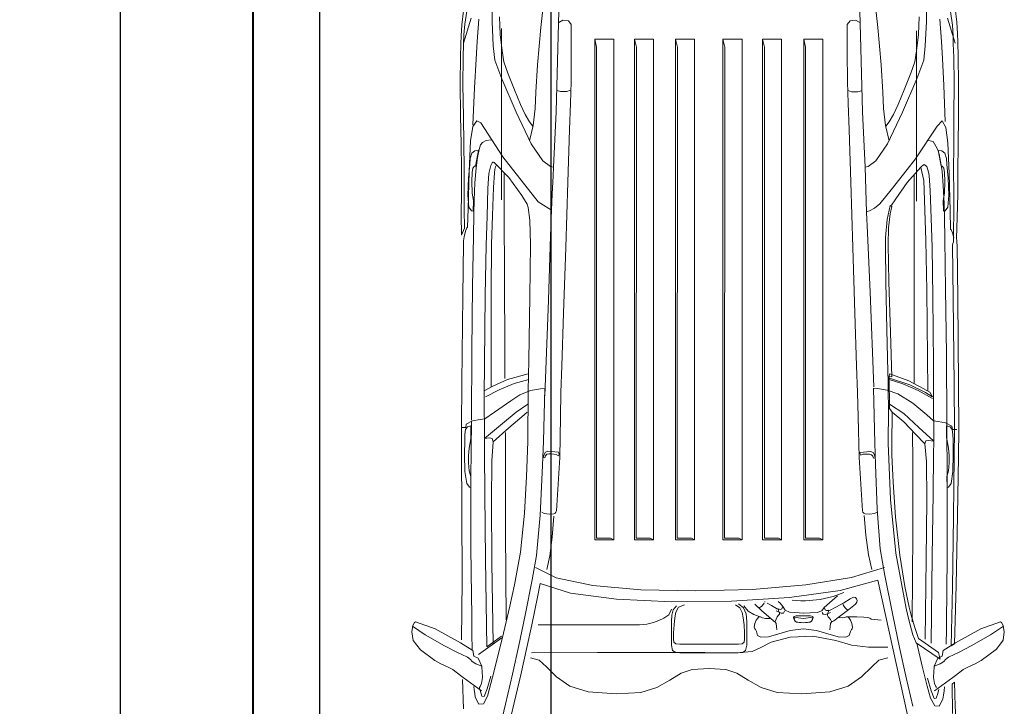
# Model space of a CAD drawing. Units: inches. Extents: x -19 to 419, y -828 to 43.
# Tile 2 of 9: x -9 to 124, y -720 to -627. Entities that reach past the tile are written whole.
import ezdxf

# ---------------------------------------------------------------- set-up
doc = ezdxf.new("R2010")
doc.units = ezdxf.units.IN
doc.header["$MEASUREMENT"] = 0
for name, color, linetype, lineweight in [('A-ANNO-DIMS', 2, 'Continuous', 18), ('A-EQPM-VEHI', 8, 'Continuous', 13), ('A-WALL', 7, 'Continuous', 40)]:
    doc.layers.add(name, color=color, linetype=linetype, lineweight=lineweight)
doc.styles.get("Standard").update_dxf_attribs({"font": 'arial.ttf'})
doc.dimstyles.get("Standard").update_dxf_attribs({"dimtxt": 0.18, "dimasz": 0.18, "dimexe": 0.18, "dimexo": 0.0625, "dimgap": 0.09, "dimtad": 0, "dimtih": 1, "dimtoh": 1, "dimdec": 0, "dimzin": 0, "dimdsep": 46, "dimlunit": 3, "dimtxsty": 'Standard', "dimcen": 0.09, "dimadec": 0, "dimazin": 0, "dimtfac": 1, "dimtdec": 0, "dimtofl": 0, "dimtmove": 0, "dimatfit": 3, "dimfxl": 1, "dimtolj": 1, "dimtzin": 0, "dimarcsym": 0})

# ---------------------------------------------------------------- blocks, each defined once
blk = doc.blocks.new('*D2')
at = {"layer": 'A-ANNO-DIMS', "color": 0, "lineweight": -2, "transparency": 16777216}
for p, q in [((22.68, 4.77), (4.74, 4.77)), ((4.92, 4.59), (4.92, -387.33)), ((4.92, -785.55), (4.92, -393.64)), ((22.68, -785.73), (4.74, -785.73))]:
    blk.add_line(p, q, dxfattribs=at)
at = {"layer": 'A-ANNO-DIMS', "color": 0, "transparency": 16777216}
for points in [[(4.89, 4.59), (4.95, 4.59), (4.92, 4.77)], [(4.89, -785.55), (4.95, -785.55), (4.92, -785.73)]]:
    blk.add_solid(points, dxfattribs=at)
at = {"layer": 'Defpoints', "color": 0, "transparency": 16777216}
for p in [(22.74, 4.77), (4.92, -785.73), (22.74, -785.73)]:
    blk.add_point(p, dxfattribs=at)
at = {"layer": 'A-ANNO-DIMS', "color": 0, "transparency": 16777216, "insert": (4.92, -390.48), "char_height": 6, "attachment_point": 5}
blk.add_mtext('\\A1;65\'-11"', dxfattribs=at)
blk = doc.blocks.new('*D49')
at = {"layer": 'A-ANNO-DIMS', "color": 0, "lineweight": -2, "transparency": 16777216}
for p, q in [((31.74, -574.3), (31.74, -827.51)), ((62.91, -574.3), (62.91, -827.51)), ((31.92, -827.33), (46.99, -827.33)), ((62.73, -827.33), (47.65, -827.33))]:
    blk.add_line(p, q, dxfattribs=at)
at = {"layer": 'A-ANNO-DIMS', "color": 0, "transparency": 16777216}
for points in [[(31.92, -827.3), (31.92, -827.36), (31.74, -827.33)], [(62.73, -827.3), (62.73, -827.36), (62.91, -827.33)]]:
    blk.add_solid(points, dxfattribs=at)
at = {"layer": 'Defpoints', "color": 0, "transparency": 16777216}
for p in [(31.74, -574.23), (62.91, -574.23), (62.91, -827.33)]:
    blk.add_point(p, dxfattribs=at)
at = {"layer": 'A-ANNO-DIMS', "color": 0, "transparency": 16777216, "insert": (47.32, -827.33), "char_height": 0.18, "attachment_point": 5}
blk.add_mtext('\\A1;2\'-7"', dxfattribs=at)

msp = doc.modelspace()

# ---------------------------------------------------------------- linework, layer by layer
at = {"layer": 'A-EQPM-VEHI'}
for p, q in [((55.01, -627.49), (55.03, -624.8)), ((113.5, -627.49), (113.48, -624.8)), ((50.91, -627.91), (51.15, -626.02)), ((51.59, -626.09), (51.31, -627.85)), ((61.53, -628.28), (61.9, -625.06)), ((63.86, -631.09), (63.96, -626.08)), ((104.65, -631.09), (104.55, -626.08)), ((106.97, -628.28), (106.61, -625.06)), ((117.01, -627.96), (116.77, -626.12)), ((117.37, -625.69), (117.61, -627.58)), ((51.11, -630.39), (52.17, -627.01)), ((52.97, -630.19), (53.18, -627.18)), ((55.15, -630.74), (55.01, -627.49)), ((56.07, -629.23), (55.99, -626.85)), ((63.96, -627.62), (64.51, -627.28)), ((64.51, -627.28), (65.27, -627.39)), ((65.27, -627.39), (65.65, -627.86)), ((103.22, -627.39), (102.84, -627.86)), ((103.97, -627.28), (103.22, -627.39)), ((104.52, -627.62), (103.97, -627.28)), ((112.44, -629.23), (112.51, -626.85)), ((113.35, -630.74), (113.5, -627.49)), ((115.53, -630.19), (115.32, -627.18)), ((117.4, -630.39), (116.34, -627.01)), ((50.81, -629.42), (50.91, -627.91)), ((51.31, -627.85), (51.19, -629.27)), ((56.23, -651.51), (56.23, -628.43)), ((61.11, -633.31), (61.53, -628.28)), ((65.65, -627.86), (65.65, -631.57)), ((102.84, -627.86), (102.84, -631.57)), ((107.4, -633.31), (106.97, -628.28)), ((112.17, -651.67), (112.17, -628.72)), ((117.1, -629.42), (117.01, -627.96)), ((117.61, -627.58), (117.71, -629.09)), ((50.78, -630.5), (50.81, -629.42)), ((51.19, -629.27), (51.15, -630.43)), ((56.32, -631.45), (56.07, -629.23)), ((68.82, -629.87), (71.39, -629.87)), ((68.82, -697.34), (68.82, -629.87)), ((68.82, -629.87), (69.07, -630.94)), ((71.39, -629.87), (71.39, -697.34)), ((74.16, -697.34), (74.16, -629.87)), ((74.16, -629.87), (76.73, -629.87)), ((74.16, -697.34), (74.16, -629.87)), ((74.16, -629.87), (74.42, -630.94)), ((76.73, -629.87), (76.73, -697.34)), ((79.7, -697.34), (79.7, -629.87)), ((79.7, -629.87), (82.27, -629.87)), ((79.7, -697.34), (79.7, -629.87)), ((79.7, -629.87), (79.96, -630.94)), ((82.27, -629.87), (82.27, -697.34)), ((86.09, -697.34), (86.09, -629.87)), ((86.09, -629.87), (88.66, -629.87)), ((86.09, -697.34), (86.09, -629.87)), ((86.09, -629.87), (86.35, -630.94)), ((88.66, -629.87), (88.66, -697.34)), ((91.43, -697.34), (91.43, -629.87)), ((91.43, -629.87), (94, -629.87)), ((91.43, -697.34), (91.43, -629.87)), ((91.43, -629.87), (91.69, -630.94)), ((94, -629.87), (94, -697.34)), ((96.97, -697.34), (96.97, -629.87)), ((96.97, -629.87), (99.54, -629.87)), ((96.97, -697.34), (96.97, -629.87)), ((96.97, -629.87), (97.23, -630.94)), ((99.54, -629.87), (99.54, -697.34)), ((112.19, -631.45), (112.44, -629.23)), ((117.13, -630.5), (117.1, -629.42)), ((117.71, -629.09), (117.74, -630.26)), ((50.72, -632.26), (50.78, -630.5)), ((51.15, -630.43), (51.09, -632.36)), ((52.83, -632.56), (52.97, -630.19)), ((55.35, -632.7), (55.15, -630.74)), ((56.57, -632.89), (56.32, -631.45)), ((63.6, -639.64), (63.86, -631.09)), ((69.07, -630.94), (69.05, -697.12)), ((74.42, -630.94), (74.39, -697.12)), ((79.96, -630.94), (79.93, -697.12)), ((86.35, -630.94), (86.32, -697.12)), ((91.69, -630.94), (91.67, -697.12)), ((97.23, -630.94), (97.2, -697.12)), ((104.9, -639.64), (104.65, -631.09)), ((111.94, -632.89), (112.19, -631.45)), ((113.16, -632.7), (113.35, -630.74)), ((115.65, -632.44), (115.53, -630.19)), ((117.2, -632.26), (117.13, -630.5)), ((117.74, -630.26), (117.79, -632.18)), ((50.68, -635.78), (50.72, -632.26)), ((51.09, -632.36), (51.06, -635.97)), ((52.6, -636.43), (52.83, -632.56)), ((56.3, -635.18), (55.35, -632.7)), ((65.65, -631.57), (65.62, -635.6)), ((102.84, -631.57), (102.87, -635.6)), ((112.21, -635.18), (113.16, -632.7)), ((115.83, -636.1), (115.65, -632.44)), ((117.23, -635.78), (117.2, -632.26)), ((117.79, -632.18), (117.82, -635.78)), ((57.11, -634.42), (56.57, -632.89)), ((60.87, -637), (61.11, -633.31)), ((107.63, -637), (107.4, -633.31)), ((111.4, -634.42), (111.94, -632.89)), ((58.21, -639.7), (56.3, -635.18)), ((58.02, -636.67), (57.11, -634.42)), ((110.3, -639.7), (112.21, -635.18)), ((110.49, -636.67), (111.4, -634.42)), ((50.73, -640.19), (50.68, -635.78)), ((51.06, -635.97), (51.11, -640.31)), ((52.37, -641.41), (52.6, -636.43)), ((58.82, -638.67), (58.02, -636.67)), ((63.74, -636.76), (64.2, -636.91)), ((65.07, -636.9), (65.53, -636.72)), ((65.62, -635.6), (65.54, -638.48)), ((102.87, -635.6), (102.94, -638.48)), ((103.42, -636.95), (102.96, -636.77)), ((109.69, -638.67), (110.49, -636.67)), ((116.03, -640.97), (115.83, -636.1)), ((117.21, -640.24), (117.23, -635.78)), ((117.82, -635.78), (117.81, -640.24)), ((60.77, -639.19), (60.87, -637)), ((64.2, -636.91), (65.07, -636.9)), ((104.28, -636.96), (103.42, -636.95)), ((104.75, -636.81), (104.28, -636.96)), ((107.74, -639.19), (107.63, -637)), ((59.42, -640.02), (58.82, -638.67)), ((60.53, -641.5), (60.77, -639.19)), ((65.54, -638.48), (65.41, -642.06)), ((102.94, -638.48), (103.08, -642.06)), ((107.98, -641.5), (107.74, -639.19)), ((109.08, -640.02), (109.69, -638.67)), ((50.82, -644.01), (50.73, -640.19)), ((51.11, -640.31), (51.19, -643.98)), ((60.23, -643.94), (58.21, -639.7)), ((60.01, -640.98), (59.42, -640.02)), ((63.25, -647.09), (63.6, -639.64)), ((105.26, -647.09), (104.9, -639.64)), ((108.28, -643.94), (110.3, -639.7)), ((108.49, -640.98), (109.08, -640.02)), ((117.18, -644.15), (117.21, -640.24)), ((117.81, -640.24), (117.77, -644.15)), ((52.41, -641.63), (52.07, -643.55)), ((52.93, -640.84), (52.41, -641.63)), ((53.46, -641.11), (52.93, -640.84)), ((56.41, -645.72), (53.46, -641.11)), ((60.49, -641.56), (60.01, -640.98)), ((60.04, -643.55), (60.53, -641.5)), ((65.41, -642.06), (65.18, -649.13)), ((103.08, -642.06), (103.31, -649.13)), ((108.47, -643.55), (107.98, -641.5)), ((108.02, -641.56), (108.49, -640.98)), ((112.03, -646), (114.94, -641.56)), ((114.94, -641.56), (115.63, -640.86)), ((115.63, -640.86), (116.1, -641.76)), ((116.1, -641.76), (116.37, -643.83)), ((50.86, -647.35), (50.82, -644.01)), ((51.19, -643.98), (51.23, -647.25)), ((52.07, -643.55), (51.89, -647.67)), ((53.03, -645.82), (53.24, -644.73)), ((53.24, -644.73), (53.44, -644.11)), ((53.44, -644.11), (53.71, -643.76)), ((53.71, -643.76), (54.17, -643.49)), ((54.17, -643.49), (54.85, -643.44)), ((61.81, -646.24), (60.23, -643.94)), ((106.69, -646.24), (108.28, -643.94)), ((114.41, -643.66), (113.8, -643.51)), ((114.79, -644.26), (114.41, -643.66)), ((115.03, -644.78), (114.79, -644.26)), ((116.37, -643.83), (116.56, -647.94)), ((117.16, -647.54), (117.18, -644.15)), ((117.77, -644.15), (117.76, -647.54)), ((51.98, -646.7), (52.05, -645.92)), ((52.05, -645.92), (52.25, -645.23)), ((52.25, -645.23), (52.64, -644.9)), ((52.64, -644.9), (53.16, -644.8)), ((53.16, -644.8), (52.74, -646.95)), ((52.83, -647.21), (53.03, -645.82)), ((61.2, -651.79), (56.41, -645.72)), ((110.93, -647.41), (112.03, -646)), ((115.22, -645.34), (115.03, -644.78)), ((115.6, -644.9), (115.08, -644.8)), ((115.08, -644.8), (115.5, -646.95)), ((115.41, -646.33), (115.22, -645.34)), ((115.99, -645.23), (115.6, -644.9)), ((116.19, -645.92), (115.99, -645.23)), ((116.26, -646.7), (116.19, -645.92)), ((50.84, -650.51), (50.86, -647.35)), ((51.23, -647.25), (51.22, -650.18)), ((51.82, -648.59), (51.98, -646.7)), ((52.41, -647.23), (52.3, -647.82)), ((52.63, -646.99), (52.41, -647.23)), ((52.74, -646.95), (52.63, -646.99)), ((52.66, -649.2), (52.83, -647.21)), ((54.66, -647.44), (54.8, -646.88)), ((54.8, -646.88), (54.99, -646.5)), ((55.07, -646.45), (54.99, -646.5)), ((55.16, -646.44), (55.07, -646.45)), ((55.26, -646.49), (55.16, -646.44)), ((57.22, -648.51), (55.26, -646.49)), ((55.37, -647.44), (55.43, -647.08)), ((55.43, -647.08), (55.59, -646.8)), ((62.87, -647.01), (61.81, -646.24)), ((63.25, -647.09), (62.87, -647.01)), ((63.2, -648.26), (63.25, -647.09)), ((105.26, -647.09), (105.64, -647.01)), ((105.45, -653.15), (105.26, -647.09)), ((105.64, -647.01), (106.69, -646.24)), ((110.93, -649.17), (112.76, -647.1)), ((112.9, -646.98), (112.76, -647.1)), ((113.16, -648.91), (112.76, -647.15)), ((113.04, -646.86), (112.9, -646.98)), ((113.18, -646.76), (113.04, -646.86)), ((113.56, -647), (113.18, -646.76)), ((113.8, -647.78), (113.56, -647)), ((115.61, -647.66), (115.41, -646.33)), ((115.5, -646.95), (115.61, -646.99)), ((115.61, -646.99), (115.83, -647.23)), ((115.83, -647.23), (115.94, -647.82)), ((116.42, -648.59), (116.26, -646.7)), ((51.7, -650.89), (51.82, -648.59)), ((51.89, -647.67), (51.74, -652.71)), ((52.3, -647.82), (52.27, -649.05)), ((54.43, -649.96), (54.56, -647.96)), ((54.56, -647.96), (54.66, -647.44)), ((55.17, -649.86), (55.3, -647.86)), ((55.3, -647.86), (55.37, -647.44)), ((56.62, -652.95), (56.6, -647.89)), ((58.97, -650.94), (57.22, -648.51)), ((63.08, -650.73), (63.2, -648.26)), ((108.77, -650.18), (110.93, -647.41)), ((111.84, -653.28), (111.84, -648.17)), ((113.88, -648.23), (113.8, -647.78)), ((114.01, -650.23), (113.88, -648.23)), ((115.77, -649.64), (115.61, -647.66)), ((115.94, -647.82), (115.97, -649.05)), ((116.54, -650.89), (116.42, -648.59)), ((116.56, -647.94), (116.7, -652.99)), ((117.19, -650.51), (117.16, -647.54)), ((117.76, -647.54), (117.74, -650.75)), ((52.27, -649.05), (52.28, -650.6)), ((52.55, -651.57), (52.66, -649.2)), ((54.3, -653.72), (54.43, -649.96)), ((55.05, -653.62), (55.17, -649.86)), ((65.18, -649.13), (64.9, -657.95)), ((103.31, -649.13), (103.59, -657.95)), ((109.37, -651.36), (110.93, -649.17)), ((113.31, -652.92), (113.16, -648.91)), ((115.88, -652.01), (115.77, -649.64)), ((115.97, -649.05), (115.96, -650.6)), ((50.82, -653.55), (50.84, -650.51)), ((51.22, -650.18), (51.21, -652.82)), ((51.86, -652.49), (51.7, -650.89)), ((52.28, -650.6), (52.46, -651.6)), ((59.73, -652.11), (58.97, -650.94)), ((62.99, -652.89), (63.08, -650.73)), ((107.24, -652.06), (108.77, -650.18)), ((108.71, -652.38), (109.37, -651.36)), ((114.14, -654), (114.01, -650.23)), ((115.96, -650.6), (115.78, -651.6)), ((116.38, -652.49), (116.54, -650.89)), ((117.22, -653.21), (117.19, -650.51)), ((117.74, -650.75), (117.67, -653.91)), ((51.74, -652.71), (51.69, -655.17)), ((52.22, -653), (51.86, -652.49)), ((52.46, -651.6), (52.42, -653.03)), ((52.51, -653.34), (52.55, -651.57)), ((59.85, -652.56), (59.73, -652.11)), ((60.06, -654.23), (59.85, -652.56)), ((62.99, -652.89), (61.2, -651.79)), ((105.83, -652.99), (106.51, -652.65)), ((106.51, -652.65), (107.24, -652.06)), ((108.2, -654.14), (108.63, -652.29)), ((108.83, -652.39), (108.61, -653.38)), ((108.63, -652.29), (108.83, -652.39)), ((115.78, -651.6), (115.82, -653.03)), ((115.93, -653.79), (115.88, -652.01)), ((116.02, -653), (116.38, -652.49)), ((50.88, -656.29), (50.82, -653.55)), ((51.21, -652.82), (51.28, -655.33)), ((52.42, -653.03), (52.22, -653)), ((52.46, -656.46), (52.51, -653.34)), ((54.18, -657.6), (54.3, -653.72)), ((54.92, -657.5), (55.05, -653.62)), ((56.66, -662.39), (56.62, -652.95)), ((62.87, -656.34), (62.99, -652.89)), ((105.57, -655.94), (105.45, -653.15)), ((105.53, -653.1), (105.83, -652.99)), ((108.61, -653.38), (108.41, -655.28)), ((111.86, -662.83), (111.84, -653.28)), ((113.41, -656.99), (113.31, -652.92)), ((114.26, -657.87), (114.14, -654)), ((115.82, -653.03), (116.02, -653)), ((115.97, -656.91), (115.93, -653.79)), ((116.7, -652.99), (116.76, -655.45)), ((117.17, -655.75), (117.22, -653.21)), ((117.67, -653.91), (117.57, -656.7)), ((51.28, -655.33), (50.88, -656.29)), ((51.6, -655.3), (51.4, -655.73)), ((51.69, -655.17), (51.6, -655.3)), ((60.18, -657.54), (60.06, -654.23)), ((108.01, -656.58), (108.2, -654.14)), ((108.41, -655.28), (108.34, -657.51)), ((51.2, -656.51), (51.16, -656.76)), ((51.4, -655.73), (51.2, -656.51)), ((52.35, -663.12), (52.46, -656.46)), ((62.57, -665.04), (62.87, -656.34)), ((105.91, -663.97), (105.57, -655.94)), ((107.97, -657.8), (108.01, -656.58)), ((116.76, -655.45), (116.84, -655.56)), ((116.84, -655.56), (117.02, -655.95)), ((117.02, -655.95), (117.22, -656.64)), ((117.14, -656.92), (117.17, -655.75)), ((51.11, -657.34), (51.02, -664.49)), ((51.13, -657.04), (51.11, -657.34)), ((51.16, -656.76), (51.13, -657.04)), ((54.05, -664.4), (54.18, -657.6)), ((54.84, -663.98), (54.92, -657.5)), ((60.09, -664.55), (60.18, -657.54)), ((64.9, -657.95), (64.62, -666.78)), ((103.59, -657.95), (103.87, -666.78)), ((108.03, -662.59), (107.97, -657.8)), ((108.34, -657.51), (108.46, -662.56)), ((113.54, -663.73), (113.41, -656.99)), ((114.37, -664.62), (114.26, -657.87)), ((116.08, -663.56), (115.97, -656.91)), ((117.03, -657.63), (117.07, -657.38)), ((117.13, -664.78), (117.03, -657.63)), ((117.07, -657.38), (117.14, -657.16)), ((117.14, -657.16), (117.14, -656.92)), ((117.57, -656.7), (117.6, -657)), ((117.6, -657), (117.62, -657.3)), ((117.62, -657.3), (117.63, -657.6)), ((117.63, -657.6), (117.72, -664.76)), ((52.24, -671.85), (52.35, -663.12)), ((56.71, -671.5), (56.66, -662.39)), ((108.18, -668.96), (108.03, -662.59)), ((108.46, -662.56), (108.67, -669.38)), ((111.87, -676.21), (111.86, -662.83)), ((51.02, -664.49), (50.91, -676.1)), ((53.96, -673.49), (54.05, -664.4)), ((54.84, -672.46), (54.84, -663.98)), ((59.94, -673.1), (60.09, -664.55)), ((106.41, -676.72), (105.91, -663.97)), ((113.66, -672.71), (113.54, -663.73)), ((114.45, -673.62), (114.37, -664.62)), ((116.19, -672.29), (116.08, -663.56)), ((62.09, -677.9), (62.57, -665.04)), ((117.24, -676.38), (117.13, -664.78)), ((117.72, -664.76), (117.83, -676.38)), ((64.62, -666.78), (64.39, -673.86)), ((103.87, -666.78), (104.1, -673.86)), ((108.3, -674.7), (108.18, -668.96)), ((108.67, -669.38), (108.86, -675.37)), ((52.19, -681.18), (52.24, -671.85)), ((54.85, -676.68), (54.84, -672.46)), ((56.72, -675.59), (56.71, -671.5)), ((116.24, -681.62), (116.19, -672.29)), ((53.92, -678.03), (53.96, -673.49)), ((59.86, -677.26), (59.94, -673.1)), ((64.39, -673.86), (64.26, -677.47)), ((104.1, -673.86), (104.23, -677.47)), ((113.7, -677.2), (113.66, -672.71)), ((114.47, -678.11), (114.45, -673.62)), ((59.86, -674.96), (57.06, -675.74)), ((108.33, -675.95), (108.3, -674.7)), ((108.4, -675.5), (108.57, -674.97)), ((108.57, -674.97), (111.12, -675.89)), ((50.91, -676.1), (50.86, -682.18)), ((55.09, -676.6), (53.99, -677.2)), ((57.06, -675.74), (55.09, -676.6)), ((55.93, -677.12), (57.97, -676.25)), ((57.97, -676.25), (59.92, -675.73)), ((108.34, -676.76), (108.33, -675.95)), ((111.29, -676.43), (108.4, -675.5)), ((110.34, -676.3), (108.49, -675.74)), ((108.86, -675.37), (108.5, -675.32)), ((108.5, -675.32), (108.52, -679.63)), ((112.41, -677.22), (110.34, -676.3)), ((111.12, -675.89), (113.07, -676.92)), ((113.38, -677.49), (111.29, -676.43)), ((117.29, -682.47), (117.24, -676.38)), ((117.83, -676.38), (117.88, -682.47)), ((54.1, -678.05), (55.93, -677.12)), ((58.71, -677.77), (57.53, -678.59)), ((60.15, -677.18), (58.71, -677.77)), ((59.8, -684.03), (59.86, -677.26)), ((61.5, -676.97), (60.15, -677.18)), ((62.09, -676.94), (61.5, -676.97)), ((61.9, -684.03), (62.09, -676.94)), ((64.26, -677.47), (64.21, -680.77)), ((104.23, -677.47), (104.29, -680.77)), ((106.54, -684.31), (106.39, -676.89)), ((106.39, -676.89), (106.93, -676.94)), ((106.93, -676.94), (108.21, -677.16)), ((108.21, -677.16), (109.67, -677.64)), ((108.35, -677.05), (108.34, -676.76)), ((108.38, -679.87), (108.35, -677.05)), ((109.67, -677.64), (111.67, -678.92)), ((114.33, -678.29), (112.41, -677.22)), ((113.07, -676.92), (113.98, -677.44)), ((114.32, -678.04), (113.38, -677.49)), ((113.98, -677.44), (114.32, -678.04)), ((53.94, -683.69), (53.92, -678.03)), ((57.53, -678.59), (55.31, -680.13)), ((58.23, -680.11), (59.79, -679.05)), ((110.46, -680.31), (108.51, -679.03)), ((111.67, -678.92), (113.54, -680.46)), ((114.5, -684.05), (114.47, -678.11)), ((55.31, -680.13), (54, -681.03)), ((56.1, -681.87), (58.23, -680.11)), ((59, -680.74), (59.73, -680.14)), ((108.35, -684.31), (108.38, -679.87)), ((108.52, -679.63), (108.87, -680.12)), ((108.87, -680.12), (108.83, -684.47)), ((110.47, -681.41), (108.87, -680.12)), ((112.48, -682.18), (110.46, -680.31)), ((113.54, -680.46), (114.47, -681.28)), ((51.5, -681.73), (51.43, -682.18)), ((52.36, -681.3), (51.5, -681.73)), ((52.13, -689.08), (52.2, -681.35)), ((53.4, -681.13), (52.36, -681.3)), ((54, -681.03), (53.4, -681.13)), ((53.94, -683.69), (56.1, -681.87)), ((57.25, -682.23), (59, -680.74)), ((64.21, -680.77), (64.1, -686.25)), ((104.29, -680.77), (104.44, -686.25)), ((112.03, -683.09), (110.47, -681.41)), ((114.47, -681.28), (115.07, -681.38)), ((115.07, -681.38), (116.09, -681.56)), ((116.09, -681.56), (116.95, -682.01)), ((116.31, -689.35), (116.24, -681.62)), ((50.88, -685.49), (50.86, -682.18)), ((51.43, -682.18), (50.88, -682.18)), ((51.29, -683.91), (51.31, -683.13)), ((51.31, -683.13), (51.41, -682.44)), ((51.41, -682.44), (51.68, -682.1)), ((51.68, -682.1), (52.14, -681.97)), ((52.14, -681.97), (52.14, -683.54)), ((55.13, -684.1), (57.25, -682.23)), ((56.78, -686.7), (56.79, -682.88)), ((111.66, -686.77), (111.65, -682.88)), ((113.31, -684.37), (112.03, -683.09)), ((114.5, -684.05), (112.48, -682.18)), ((116.7, -682.1), (116.23, -681.97)), ((116.23, -681.97), (116.23, -683.54)), ((116.97, -682.44), (116.7, -682.1)), ((116.95, -682.01), (117.01, -682.45)), ((117.07, -683.13), (116.97, -682.44)), ((117.01, -682.45), (117.59, -682.47)), ((117.09, -683.91), (117.07, -683.13)), ((117.26, -686.13), (117.29, -682.47)), ((117.88, -682.47), (117.83, -686.09)), ((51.26, -685.81), (51.29, -683.91)), ((52.06, -683.99), (51.91, -684.99)), ((52.14, -683.54), (52.06, -683.99)), ((54.63, -683.59), (53.94, -683.69)), ((53.96, -685.61), (53.94, -683.69)), ((55, -683.69), (54.63, -683.59)), ((54.94, -686.66), (55.13, -684.1)), ((55.13, -684.1), (55, -683.69)), ((59.75, -685.34), (59.8, -684.03)), ((61.78, -687.31), (61.9, -684.03)), ((106.63, -687.18), (106.54, -684.31)), ((108.67, -691.87), (108.35, -684.31)), ((108.83, -684.47), (108.86, -685.93)), ((113.31, -684.37), (113.44, -683.99)), ((113.51, -686.79), (113.31, -684.37)), ((113.44, -683.99), (113.8, -683.92)), ((113.8, -683.92), (114.5, -684.05)), ((114.47, -685.83), (114.5, -684.05)), ((116.23, -683.54), (116.32, -683.99)), ((116.32, -683.99), (116.47, -684.99)), ((117.11, -685.81), (117.09, -683.91)), ((50.92, -693.38), (50.88, -685.49)), ((51.31, -688.12), (51.26, -685.81)), ((51.91, -684.99), (51.82, -685.96)), ((54.01, -691.14), (53.96, -685.61)), ((59.61, -688.81), (59.75, -685.34)), ((61.99, -685.83), (61.88, -686.24)), ((62.18, -685.49), (61.99, -685.83)), ((62.51, -685.37), (62.18, -685.49)), ((62.2, -686.02), (62.37, -685.8)), ((62.37, -685.8), (62.64, -685.73)), ((63.95, -685.51), (62.51, -685.37)), ((62.64, -685.73), (62.98, -685.75)), ((62.98, -685.75), (63.61, -685.84)), ((63.61, -685.84), (63.95, -686.01)), ((63.98, -685.6), (63.95, -685.51)), ((63.95, -686.01), (64.02, -685.81)), ((64.02, -685.81), (63.98, -685.6)), ((104.54, -685.56), (105.98, -685.42)), ((104.54, -685.61), (104.54, -685.56)), ((104.58, -685.74), (104.54, -685.61)), ((104.69, -685.91), (104.58, -685.74)), ((104.98, -685.78), (104.69, -685.91)), ((105.55, -685.77), (104.98, -685.78)), ((105.85, -685.78), (105.55, -685.77)), ((106.11, -685.85), (105.85, -685.78)), ((105.98, -685.42), (106.31, -685.54)), ((106.29, -686.07), (106.11, -685.85)), ((106.31, -685.54), (106.5, -685.88)), ((106.5, -685.88), (106.61, -686.29)), ((114.41, -691.06), (114.47, -685.83)), ((116.47, -684.99), (116.55, -685.96)), ((117.07, -688.12), (117.11, -685.81)), ((51.82, -685.96), (51.82, -686.94)), ((51.82, -686.94), (51.88, -688.03)), ((54.89, -692.15), (54.94, -686.66)), ((56.79, -696.12), (56.78, -686.7)), ((61.88, -686.24), (62.1, -686.28)), ((62.1, -686.28), (62.2, -686.02)), ((64.1, -686.25), (63.65, -693.44)), ((104.44, -686.25), (104.9, -693.44)), ((106.39, -686.33), (106.29, -686.07)), ((106.61, -686.29), (106.39, -686.33)), ((106.89, -693.21), (106.63, -687.18)), ((108.86, -685.93), (109.01, -689.56)), ((111.66, -696.32), (111.66, -686.77)), ((113.56, -691.96), (113.51, -686.79)), ((116.56, -686.94), (116.5, -688.03)), ((116.55, -685.96), (116.56, -686.94)), ((117.17, -694.21), (117.26, -686.13)), ((117.83, -686.09), (117.7, -694.06)), ((51.56, -689.72), (51.31, -688.12)), ((51.88, -688.03), (52.11, -688.77)), ((61.45, -694.01), (61.78, -687.31)), ((116.5, -688.03), (116.27, -688.77)), ((116.82, -689.72), (117.07, -688.12)), ((51.92, -690.24), (51.56, -689.72)), ((52.11, -688.77), (52.1, -690.28)), ((52.12, -691.97), (52.13, -689.08)), ((59.35, -693.74), (59.61, -688.81)), ((109.01, -689.56), (109.33, -694.26)), ((116.27, -688.77), (116.28, -690.28)), ((116.32, -692.25), (116.31, -689.35)), ((116.46, -690.24), (116.82, -689.72)), ((52.1, -690.28), (51.92, -690.24)), ((54.11, -699.97), (54.01, -691.14)), ((114.29, -699.59), (114.41, -691.06)), ((116.28, -690.28), (116.46, -690.24)), ((52.12, -698.38), (52.12, -691.97)), ((54.97, -700.43), (54.89, -692.15)), ((109.38, -699.14), (108.67, -691.87)), ((113.49, -699.92), (113.56, -691.96)), ((116.32, -698.65), (116.32, -692.25)), ((50.93, -702.83), (50.92, -693.38)), ((58.79, -698.98), (59.35, -693.74)), ((62.02, -693.79), (61.67, -693.59)), ((62.7, -693.86), (62.02, -693.79)), ((63.31, -693.8), (62.7, -693.86)), ((63.47, -693.73), (63.31, -693.8)), ((63.59, -693.6), (63.47, -693.73)), ((63.65, -693.44), (63.59, -693.6)), ((104.9, -693.44), (104.96, -693.6)), ((104.96, -693.6), (105.08, -693.73)), ((105.08, -693.73), (105.24, -693.8)), ((105.24, -693.8), (105.85, -693.86)), ((105.85, -693.86), (106.53, -693.79)), ((106.53, -693.79), (106.88, -693.59)), ((107.29, -698.53), (106.89, -693.21)), ((60.99, -699.42), (61.45, -694.01)), ((63.07, -696.98), (63.3, -694.14)), ((105.33, -696.71), (105.1, -694.04)), ((109.33, -694.26), (109.92, -699.39)), ((117.03, -703.7), (117.17, -694.21)), ((117.7, -694.06), (117.52, -703.46)), ((56.86, -708.1), (56.79, -696.12)), ((111.58, -708.38), (111.66, -696.32)), ((62.75, -699.47), (63.07, -696.98)), ((71.39, -697.34), (68.82, -697.34)), ((69.05, -697.12), (70.95, -697.12)), ((70.95, -697.12), (71.39, -697.34)), ((74.16, -697.34), (76.73, -697.34)), ((74.39, -697.12), (76.3, -697.12)), ((76.3, -697.12), (76.73, -697.34)), ((79.7, -697.34), (82.27, -697.34)), ((79.93, -697.12), (81.84, -697.12)), ((81.84, -697.12), (82.27, -697.34)), ((86.09, -697.34), (88.66, -697.34)), ((86.32, -697.12), (88.23, -697.12)), ((88.23, -697.12), (88.66, -697.34)), ((91.43, -697.34), (94.01, -697.34)), ((91.67, -697.12), (93.57, -697.12)), ((93.57, -697.12), (94.01, -697.34)), ((96.97, -697.34), (99.55, -697.34)), ((97.2, -697.12), (99.11, -697.12)), ((99.11, -697.12), (99.55, -697.34)), ((105.7, -699.35), (105.33, -696.71)), ((52.2, -704.85), (52.12, -698.38)), ((58.01, -703.39), (58.79, -698.98)), ((107.91, -702.11), (107.29, -698.53)), ((110.78, -706.6), (109.38, -699.14)), ((116.24, -705.12), (116.32, -698.65)), ((54.27, -711.76), (54.11, -699.97)), ((55.13, -711.36), (54.97, -700.43)), ((60.39, -702.7), (60.99, -699.42)), ((62.35, -701.31), (62.75, -699.47)), ((106.14, -701.31), (105.7, -699.35)), ((109.92, -699.39), (110.61, -703.61)), ((113.34, -710.7), (113.49, -699.92)), ((114.13, -711.24), (114.29, -699.59)), ((60.84, -701.04), (63.6, -702.46)), ((103.41, -702.4), (107.86, -701.04)), ((50.84, -710.8), (50.93, -702.83)), ((59.43, -707.49), (60.39, -702.7)), ((63.6, -702.46), (68.55, -703.46)), ((97.26, -703.39), (103.41, -702.4)), ((106.96, -702.78), (101.87, -704.14)), ((110.98, -721.14), (106.96, -702.78)), ((108.96, -707.47), (107.91, -702.11)), ((57.37, -706.25), (58.01, -703.39)), ((61.47, -703.22), (61.1, -705.03)), ((65.56, -704.5), (61.47, -703.22)), ((68.55, -703.46), (75.04, -704.05)), ((75.04, -704.05), (82.42, -704.22)), ((82.42, -704.22), (90.05, -704)), ((90.05, -704), (97.26, -703.39)), ((101.87, -704.14), (95.04, -705.08)), ((102.37, -704.41), (100.94, -704.98)), ((110.61, -703.61), (111.18, -706.38)), ((116.84, -711.63), (117.03, -703.7)), ((117.52, -703.46), (117.31, -711.35)), ((52.24, -707.44), (52.2, -704.85)), ((61.1, -705.03), (60.32, -708.76)), ((71.73, -705.32), (65.56, -704.5)), ((79.2, -705.68), (71.73, -705.32)), ((87.23, -705.6), (79.2, -705.68)), ((95.04, -705.08), (87.23, -705.6)), ((91.71, -705.69), (91.74, -705.69)), ((91.8, -705.69), (91.71, -705.69)), ((91.74, -705.69), (91.77, -705.69)), ((91.77, -705.69), (91.8, -705.69)), ((93.78, -705.88), (93.54, -705.62)), ((96.01, -705.51), (95.42, -705.44)), ((96.57, -705.53), (96.01, -705.51)), ((97.2, -705.53), (96.57, -705.53)), ((99.17, -705.38), (97.2, -705.53)), ((100.94, -704.98), (99.17, -705.38)), ((100.45, -705.8), (101.18, -705.18)), ((101.18, -705.18), (101.52, -704.89)), ((103.22, -705.29), (102.38, -705.8)), ((103.66, -705.07), (103.22, -705.29)), ((103.94, -705.1), (103.66, -705.07)), ((104.09, -705.27), (103.94, -705.1)), ((103.96, -706), (104.13, -705.74)), ((104.17, -705.49), (104.09, -705.27)), ((104.13, -705.74), (104.17, -705.49)), ((116.21, -707.44), (116.24, -705.12)), ((56.51, -709.89), (57.37, -706.25)), ((78.79, -707.42), (79.16, -706.67)), ((79.4, -706.78), (79.2, -707.49)), ((79.81, -706.24), (79.4, -706.78)), ((79.6, -707.82), (79.76, -707.06)), ((79.76, -707.06), (80.12, -706.42)), ((80.12, -706.42), (80.92, -706.09)), ((88.38, -706.49), (87.78, -706.08)), ((88.88, -706.51), (88.2, -705.97)), ((88.68, -707.13), (88.38, -706.49)), ((89.2, -707.31), (88.88, -706.51)), ((89.5, -706.96), (88.92, -706.2)), ((90.24, -707.38), (89.5, -706.96)), ((91.29, -706.83), (90.39, -706)), ((90.88, -706.4), (91.01, -706.45)), ((91.01, -706.45), (91.14, -706.41)), ((91.14, -706.41), (91.31, -706.26)), ((92.27, -707.71), (91.29, -706.83)), ((91.31, -706.26), (91.43, -706.11)), ((91.43, -706.11), (91.55, -705.98)), ((91.55, -705.98), (91.63, -705.84)), ((92.06, -705.84), (92.61, -706.18)), ((92.61, -706.18), (93.08, -706.45)), ((93.08, -706.45), (93.43, -706.65)), ((93.92, -707.23), (93.28, -706.91)), ((93.43, -706.65), (93.45, -706.64)), ((93.45, -706.64), (93.53, -706.64)), ((93.53, -706.64), (93.67, -706.67)), ((93.56, -706.7), (93.56, -706.67)), ((93.58, -706.8), (93.56, -706.7)), ((93.64, -706.98), (93.58, -706.8)), ((93.7, -707.17), (93.64, -706.98)), ((93.67, -706.67), (93.86, -706.7)), ((93.97, -706.09), (93.78, -705.88)), ((93.86, -706.7), (94.04, -706.61)), ((94.17, -706.31), (93.97, -706.09)), ((94.04, -706.61), (94.17, -706.31)), ((94.48, -706.79), (94.17, -706.31)), ((94.4, -706.96), (94.25, -707.2)), ((95.07, -707.09), (94.48, -706.79)), ((96.97, -707.19), (95.07, -707.09)), ((98.79, -707.12), (99.4, -706.89)), ((99.4, -706.89), (99.74, -706.45)), ((99.48, -707.1), (99.61, -707.34)), ((99.74, -706.45), (100.45, -705.8)), ((99.85, -706.77), (99.74, -706.45)), ((100.02, -706.86), (99.85, -706.77)), ((99.94, -707.38), (100.59, -707.1)), ((100.21, -706.84), (100.02, -706.86)), ((100.36, -706.82), (100.21, -706.84)), ((100.23, -707.15), (100.3, -706.98)), ((100.3, -706.98), (100.33, -706.88)), ((100.33, -706.88), (100.33, -706.84)), ((100.44, -706.83), (100.36, -706.82)), ((100.46, -706.83), (100.44, -706.83)), ((101.29, -706.41), (100.46, -706.83)), ((102.38, -705.8), (101.29, -706.41)), ((101.79, -707.66), (103.07, -706.71)), ((102.28, -706.1), (102.25, -705.89)), ((102.42, -706.32), (102.28, -706.1)), ((102.6, -706.55), (102.42, -706.32)), ((102.76, -706.72), (102.6, -706.55)), ((102.89, -706.76), (102.76, -706.72)), ((103.01, -706.72), (102.89, -706.76)), ((103.07, -706.71), (103.96, -706)), ((111.15, -708.12), (110.78, -706.6)), ((111.18, -706.38), (111.46, -707.47)), ((44.54, -708.47), (44.66, -708.38)), ((44.66, -708.38), (47.31, -709.3)), ((52.26, -709.9), (52.24, -707.44)), ((58.58, -711.55), (59.43, -707.49)), ((76.73, -708.45), (77.45, -708.18)), ((77.45, -708.18), (78.14, -707.89)), ((78.14, -707.89), (78.79, -707.42)), ((79.2, -707.49), (79.14, -708.31)), ((79.14, -708.31), (79.14, -711.53)), ((79.5, -708.78), (79.6, -707.82)), ((88.83, -707.82), (88.68, -707.13)), ((88.93, -708.78), (88.83, -707.82)), ((89.29, -708.31), (89.2, -707.31)), ((89.29, -711.53), (89.29, -708.31)), ((90.95, -707.64), (90.24, -707.38)), ((90.58, -708.17), (90.38, -708.59)), ((90.77, -707.88), (90.58, -708.17)), ((90.89, -707.74), (90.77, -707.88)), ((91, -707.69), (90.89, -707.74)), ((91.15, -707.72), (91, -707.69)), ((91.41, -707.82), (91.15, -707.72)), ((91.84, -707.92), (91.41, -707.82)), ((92.41, -707.93), (91.84, -707.92)), ((92.84, -708.21), (92.27, -707.71)), ((92.99, -708.32), (92.84, -708.21)), ((93.05, -708.33), (92.99, -708.32)), ((93.07, -708.31), (93.05, -708.33)), ((93.25, -708.6), (93.07, -708.31)), ((93.13, -708.31), (93.25, -708.01)), ((93.25, -708.01), (93.41, -707.72)), ((93.41, -707.72), (93.58, -707.5)), ((93.58, -707.5), (93.69, -707.34)), ((93.69, -707.34), (93.7, -707.17)), ((94.25, -707.2), (93.92, -707.23)), ((95.59, -707.81), (95.67, -707.65)), ((95.68, -708.08), (95.59, -707.81)), ((95.67, -707.65), (95.97, -707.59)), ((95.67, -707.94), (95.76, -707.82)), ((95.68, -708.08), (95.67, -707.94)), ((95.83, -708.3), (95.68, -708.08)), ((95.76, -707.82), (95.97, -707.8)), ((96, -708.4), (95.83, -708.3)), ((95.97, -707.59), (97.88, -707.59)), ((95.97, -707.8), (96.26, -707.85)), ((96.17, -708.44), (96, -708.4)), ((96.26, -707.85), (96.59, -707.9)), ((96.59, -707.9), (96.91, -707.91)), ((96.88, -707.19), (98.79, -707.12)), ((96.91, -707.91), (97.24, -707.9)), ((97.24, -707.9), (97.58, -707.85)), ((97.58, -707.85), (97.88, -707.8)), ((97.85, -708.4), (97.68, -708.44)), ((98.02, -708.3), (97.85, -708.4)), ((97.88, -707.59), (98.18, -707.65)), ((97.88, -707.8), (98.09, -707.82)), ((98.17, -708.08), (98.02, -708.3)), ((98.09, -707.82), (98.18, -707.94)), ((98.26, -707.81), (98.17, -708.08)), ((98.18, -707.94), (98.17, -708.08)), ((98.18, -707.65), (98.26, -707.81)), ((99.61, -707.34), (99.94, -707.38)), ((100.16, -707.34), (100.23, -707.15)), ((100.16, -707.51), (100.16, -707.34)), ((100.27, -707.68), (100.16, -707.51)), ((100.43, -707.86), (100.27, -707.68)), ((100.6, -708.06), (100.43, -707.86)), ((100.59, -708.59), (100.78, -708.31)), ((100.71, -708.31), (100.6, -708.06)), ((100.78, -708.31), (100.79, -708.33)), ((100.79, -708.33), (100.85, -708.33)), ((100.85, -708.33), (101.01, -708.23)), ((101.01, -708.23), (101.79, -707.66)), ((101.67, -707.8), (102.18, -707.82)), ((102.18, -707.82), (102.5, -707.78)), ((102.5, -707.78), (102.71, -707.72)), ((102.71, -707.72), (102.85, -707.69)), ((102.71, -707.72), (104.13, -707.72)), ((102.85, -707.69), (102.96, -707.74)), ((102.96, -707.74), (103.08, -707.88)), ((103.08, -707.88), (103.27, -708.17)), ((103.27, -708.17), (103.47, -708.59)), ((104.13, -707.72), (105.07, -707.75)), ((105.07, -707.75), (105.59, -707.79)), ((105.59, -707.79), (105.86, -707.87)), ((105.86, -707.87), (106, -707.98)), ((106, -707.98), (106.04, -708.03)), ((106.04, -708.03), (107.4, -708.13)), ((109.86, -711.83), (108.96, -707.47)), ((111.69, -710.12), (111.15, -708.12)), ((111.46, -707.47), (111.9, -709.01)), ((116.2, -709.36), (116.21, -707.44)), ((123.49, -708.38), (120.83, -709.3)), ((123.61, -708.47), (123.49, -708.38)), ((44.15, -709.72), (44.31, -708.86)), ((44.36, -710.89), (44.15, -709.72)), ((45.98, -710.14), (44.27, -708.95)), ((44.31, -708.86), (44.54, -708.47)), ((47.31, -709.3), (50.71, -711.21)), ((60.32, -708.76), (59.67, -711.85)), ((61.18, -708.78), (74.83, -708.78)), ((74.83, -708.78), (75.85, -708.68)), ((75.85, -708.68), (76.73, -708.45)), ((79.44, -709.88), (79.5, -708.78)), ((88.99, -709.88), (88.93, -708.78)), ((90.38, -708.59), (90.31, -709.08)), ((90.31, -709.08), (90.37, -709.34)), ((90.37, -709.34), (90.46, -709.39)), ((90.46, -709.39), (90.59, -709.7)), ((90.59, -709.7), (90.75, -710.2)), ((93.32, -709.02), (93.25, -708.6)), ((93.35, -709.46), (93.32, -709.02)), ((93.64, -710), (95.15, -709.53)), ((95.15, -709.53), (96.93, -709.31)), ((96.38, -708.47), (96.17, -708.44)), ((96.64, -708.48), (96.38, -708.47)), ((96.93, -708.49), (96.64, -708.48)), ((97.21, -708.48), (96.93, -708.49)), ((98.7, -709.53), (96.93, -709.31)), ((97.47, -708.47), (97.21, -708.48)), ((97.68, -708.44), (97.47, -708.47)), ((100.21, -710), (98.7, -709.53)), ((100.51, -709.46), (100.52, -709.02)), ((100.52, -709.02), (100.59, -708.59)), ((103.26, -709.7), (103.1, -710.2)), ((103.39, -709.39), (103.26, -709.7)), ((103.49, -709.34), (103.39, -709.39)), ((103.47, -708.59), (103.54, -709.08)), ((103.54, -709.08), (103.49, -709.34)), ((111.9, -709.01), (112.42, -710.61)), ((116.18, -711.4), (116.2, -709.36)), ((120.83, -709.3), (117.43, -711.21)), ((122.16, -710.14), (123.87, -708.95)), ((123.84, -708.86), (123.61, -708.47)), ((124, -709.72), (123.84, -708.86)), ((123.85, -710.85), (124, -709.72)), ((45.32, -712.15), (44.36, -710.89)), ((48.59, -711.6), (45.98, -710.14)), ((52.28, -712.22), (52.26, -709.9)), ((53.16, -712.77), (56.28, -710.53)), ((56.27, -710.31), (54.27, -711.76)), ((55.27, -715), (56.51, -709.89)), ((79.42, -710.69), (79.44, -709.88)), ((79.49, -711.11), (79.42, -710.69)), ((88.94, -711.11), (89.01, -710.69)), ((89.01, -710.69), (88.99, -709.88)), ((90.75, -710.2), (91.2, -710.46)), ((91.2, -710.46), (92.23, -710.39)), ((92.23, -710.39), (93.64, -710)), ((92.58, -711.1), (95.14, -710.44)), ((95.14, -710.44), (98.22, -710.29)), ((98.22, -710.29), (101.29, -710.9)), ((101.62, -710.39), (100.21, -710)), ((101.29, -710.9), (103.39, -711.5)), ((102.65, -710.46), (101.62, -710.39)), ((103.1, -710.2), (102.65, -710.46)), ((112.12, -711.22), (111.69, -710.12)), ((112.42, -710.61), (115.14, -712.51)), ((119.55, -711.6), (122.16, -710.14)), ((122.97, -712.08), (123.85, -710.85)), ((47.28, -713.6), (45.32, -712.15)), ((50.22, -712.45), (48.59, -711.6)), ((50.71, -711.21), (52.39, -712.25)), ((52.39, -712.25), (52.52, -713.02)), ((57.72, -715.41), (58.58, -711.55)), ((59.67, -711.85), (58.84, -715.53)), ((79.14, -711.53), (79.3, -712.26)), ((79.3, -712.26), (79.72, -712.52)), ((79.74, -711.33), (79.49, -711.11)), ((80.26, -711.4), (79.74, -711.33)), ((88.17, -711.4), (80.26, -711.4)), ((87.89, -712.55), (90.01, -712.38)), ((88.17, -711.4), (88.69, -711.33)), ((88.69, -711.33), (88.94, -711.11)), ((88.72, -712.52), (89.13, -712.26)), ((89.13, -712.26), (89.29, -711.53)), ((90.01, -712.38), (91.09, -711.87)), ((91.09, -711.87), (92.58, -711.1)), ((103.39, -711.5), (105.72, -711.79)), ((105.72, -711.79), (108.29, -711.79)), ((110.72, -715.68), (109.86, -711.83)), ((115.36, -713.4), (112.12, -711.22)), ((112.94, -714.34), (112.2, -711.26)), ((115.76, -712.25), (115.63, -713.02)), ((117.43, -711.21), (115.76, -712.25)), ((117.31, -711.35), (116.84, -711.63)), ((117.93, -712.45), (119.55, -711.6)), ((120.86, -713.6), (122.97, -712.08)), ((48.08, -714.02), (47.28, -713.6)), ((50.9, -712.77), (50.22, -712.45)), ((51.65, -713.15), (50.9, -712.77)), ((52.07, -713.47), (51.65, -713.15)), ((52.3, -713.74), (52.07, -713.47)), ((52.78, -714.04), (52.3, -713.74)), ((53.09, -713.28), (52.52, -713.02)), ((53.6, -714.36), (53.09, -713.28)), ((61.32, -713.55), (60.14, -713.24)), ((60.3, -712.54), (69.19, -712.51)), ((62.3, -714.44), (61.32, -713.55)), ((69.19, -712.51), (77.19, -712.51)), ((77.19, -712.51), (83.64, -712.53)), ((79.72, -712.52), (80.29, -712.55)), ((80.29, -712.55), (88.14, -712.55)), ((83.64, -712.53), (87.89, -712.55)), ((88.14, -712.55), (88.72, -712.52)), ((107.11, -713.55), (106.13, -714.44)), ((108.29, -713.24), (107.11, -713.55)), ((114.54, -714.36), (115.05, -713.28)), ((115.05, -713.28), (115.63, -713.02)), ((115.14, -712.51), (115.36, -713.4)), ((115.37, -714.04), (115.85, -713.74)), ((115.85, -713.74), (116.08, -713.47)), ((116.08, -713.47), (116.5, -713.15)), ((116.5, -713.15), (117.25, -712.77)), ((117.25, -712.77), (117.93, -712.45)), ((120.06, -714.02), (120.86, -713.6)), ((49.17, -714.55), (48.08, -714.02)), ((49.71, -714.81), (49.17, -714.55)), ((49.98, -715.01), (49.71, -714.81)), ((51.1, -715.86), (49.98, -715.01)), ((53.6, -714.36), (52.78, -714.04)), ((53.62, -714.55), (53.6, -714.36)), ((53.65, -715.07), (53.62, -714.55)), ((54.37, -718.38), (55.27, -715)), ((63.66, -715.78), (62.3, -714.44)), ((81.95, -714.8), (80.46, -715.29)), ((84.22, -714.65), (81.95, -714.8)), ((86.48, -714.8), (84.22, -714.65)), ((87.97, -715.29), (86.48, -714.8)), ((106.13, -714.44), (104.77, -715.78)), ((113.61, -717.03), (112.94, -714.34)), ((114.5, -715.07), (114.53, -714.55)), ((114.53, -714.55), (114.54, -714.36)), ((114.54, -714.36), (115.37, -714.04)), ((117.05, -715.86), (118.17, -715.01)), ((118.17, -715.01), (118.44, -714.81)), ((118.44, -714.81), (118.98, -714.55)), ((118.98, -714.55), (120.06, -714.02)), ((51.11, -720.09), (50.99, -716.14)), ((53.54, -717.68), (51.1, -715.86)), ((53.57, -716.67), (53.67, -715.89)), ((53.67, -715.89), (53.65, -715.07)), ((54.82, -715.7), (54.3, -717.41)), ((56.79, -719.49), (57.72, -715.41)), ((58.84, -715.53), (57.97, -719.3)), ((65.48, -717.05), (63.66, -715.78)), ((78.94, -716.23), (77.19, -717.24)), ((80.46, -715.29), (78.94, -716.23)), ((89.49, -716.23), (87.97, -715.29)), ((91.24, -717.24), (89.49, -716.23)), ((104.77, -715.78), (102.95, -717.05)), ((111.66, -719.76), (110.72, -715.68)), ((113.63, -715.98), (114.14, -717.68)), ((114.48, -715.89), (114.5, -715.07)), ((114.58, -716.67), (114.48, -715.89)), ((114.61, -717.68), (117.05, -715.86)), ((52.58, -717.56), (52.53, -717.07)), ((52.64, -718.04), (52.58, -717.56)), ((53.28, -717.23), (53.38, -717.1)), ((53.31, -717.38), (53.28, -717.23)), ((53.41, -717.77), (53.31, -717.38)), ((53.38, -717.1), (53.57, -716.67)), ((54.3, -717.41), (53.9, -718.43)), ((67.94, -717.83), (65.48, -717.05)), ((77.19, -717.24), (75.03, -717.88)), ((93.4, -717.88), (91.24, -717.24)), ((102.95, -717.05), (100.49, -717.83)), ((114.07, -718.66), (113.61, -717.03)), ((114.14, -717.68), (114.54, -718.7)), ((114.76, -717.1), (114.58, -716.67)), ((114.86, -717.23), (114.76, -717.1)), ((115.04, -718.05), (115.13, -717.65)), ((115.13, -717.65), (115.16, -717.51)), ((115.81, -718.24), (115.88, -717.68)), ((115.88, -717.68), (115.94, -717.12)), ((116.97, -716.79), (117.31, -716.49)), ((117, -720.74), (116.97, -716.79)), ((117.31, -716.49), (117.4, -719.74)), ((52.71, -718.51), (52.64, -718.04)), ((52.71, -718.51), (53.22, -719.49)), ((53.6, -718.38), (53.41, -717.77)), ((53.9, -718.43), (53.6, -718.38)), ((53.81, -719.41), (54.37, -718.38)), ((71.72, -718.1), (67.94, -717.83)), ((75.03, -717.88), (71.72, -718.1)), ((96.71, -718.1), (93.4, -717.88)), ((100.49, -717.83), (96.71, -718.1)), ((114.63, -719.68), (114.07, -718.66)), ((114.54, -718.7), (114.84, -718.66)), ((114.84, -718.66), (115.04, -718.05)), ((115.73, -718.78), (115.22, -719.76)), ((115.73, -718.78), (115.81, -718.24)), ((53.22, -719.49), (53.81, -719.41)), ((56.35, -721.38), (56.79, -719.49)), ((57.97, -719.3), (57.56, -721.02)), ((115.22, -719.76), (114.63, -719.68)), ((117.4, -719.74), (117.5, -721.96))]:
    msp.add_line(p, q, dxfattribs=at)
at = {"layer": 'A-WALL'}
msp.add_line((22.74, 4.77), (22.74, -785.73), dxfattribs=at)

# ---------------------------------------------------------------- dimensions: what is measured, and where the dimension line sits
at = {"layer": 'A-ANNO-DIMS'}
dim = msp.add_linear_dim(base=(4.917623, -785.73343372), p1=(22.73889525, 4.76656628), p2=(22.73889525, -785.73343372), angle=90, dimstyle='Standard', override={"dimtxt": 6, "dimclrd": 0, "dimclre": 0, "dimclrt": 0}, dxfattribs=at)
dim.commit()
dim.dimension.update_dxf_attribs({"geometry": '*D2', "text_midpoint": (4.917623, -390.48343372)})
dim = msp.add_linear_dim(base=(62.91, -827.33), p1=(31.74, -574.23), p2=(62.91, -574.23), dimstyle='Standard', override={"dimdec": 1, "dimlfac": 1, "dimrnd": 0, "dimzin": 1, "dimdsep": 46, "dimlunit": 4, "dimfrac": 2}, dxfattribs=at)
dim.commit()
dim.dimension.update_dxf_attribs({"geometry": '*D49', "text_midpoint": (47.32, -827.33)})

doc.saveas('drawing.dxf')
